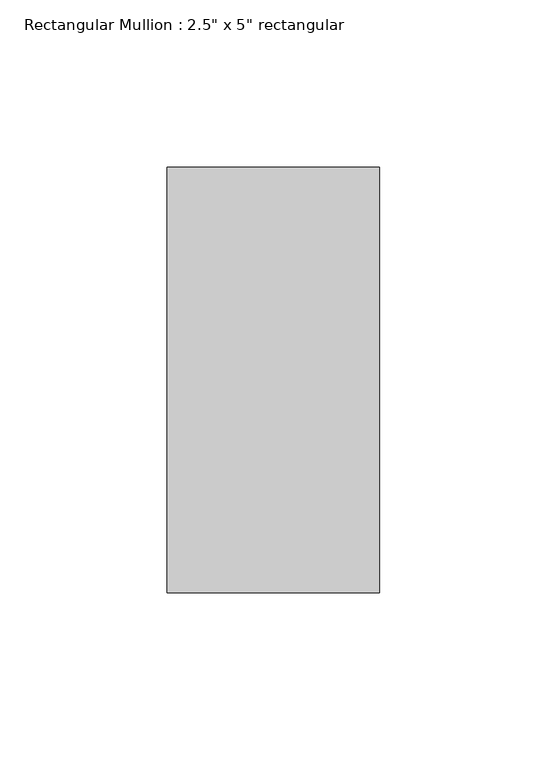
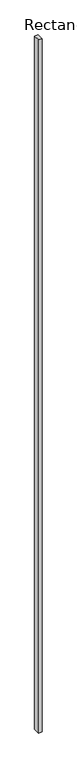
"""IFC4 building model written with IfcOpenShell, lengths in millimetres: member geometry."""

from ifc_helpers import new_model, si_unit, frame, origin, place, context, project, spatial, polyline, outline, extrude, source, transform, mapped, element, save


def member_c8d661c8(model_context):
    return source(origin(), model_context, "Body", "SweptSolid", [
        extrude(outline(polyline([(0.0, 63.5), (0.0, -63.5), (-63.5, -63.5), (-63.5, 63.5), (0.0, 63.5)])), frame((0.0, 0.0, -13705.6229265), z_axis=(0.0, 0.0, 1.0), x_axis=(1.0, 0.0, 0.0)), (0.0, 0.0, 1.0), 13705.6229265),
    ])


if __name__ == "__main__":
    model = new_model("IFC4")
    model_context = context("Model", 3, world=origin())
    ifc_project = project(units=[si_unit("LENGTHUNIT", "METRE", prefix="MILLI")], contexts=[model_context])
    site = spatial("IfcSite", under=ifc_project)
    building = spatial("IfcBuilding", under=site)
    placement = place(None, origin())
    member_shape = member_c8d661c8(model_context)
    element("IfcMember", 1, ObjectType="Rectangular Mullion : 2.5\" x 5\" rectangular", at=placement, inside=building, context=model_context, shape_type="MappedRepresentation", body=[
        mapped(member_shape, transform((0.0, 0.0, 0.0), x_axis=(1.0, 0.0, 0.0), y_axis=(0.0, 1.0, 0.0), z_axis=(0.0, 0.0, 1.0))),
    ])
    save(model, "model.ifc")

# Revit data of these elements
# Type "Rectangular Mullion : 2.5\" x 5\" rectangular"
#   built-in parameter 1007304 = 0.416667 (stored number, unit not read)
#   built-in parameter 1007301 = 0.104167 (stored number, unit not read)
#   built-in parameter 1007300 = 0.104167 (stored number, unit not read)
# Element 1 (IfcMember, "Rectangular Mullion : 2.5\" x 5\" rectangular")
#   Materials on its faces: "Aluminum"
# Materials
#   "Aluminum": class "Metal", colour RGB 247 247 247, transparency 0, Description = "Aluminum 6061", Cost = 0
